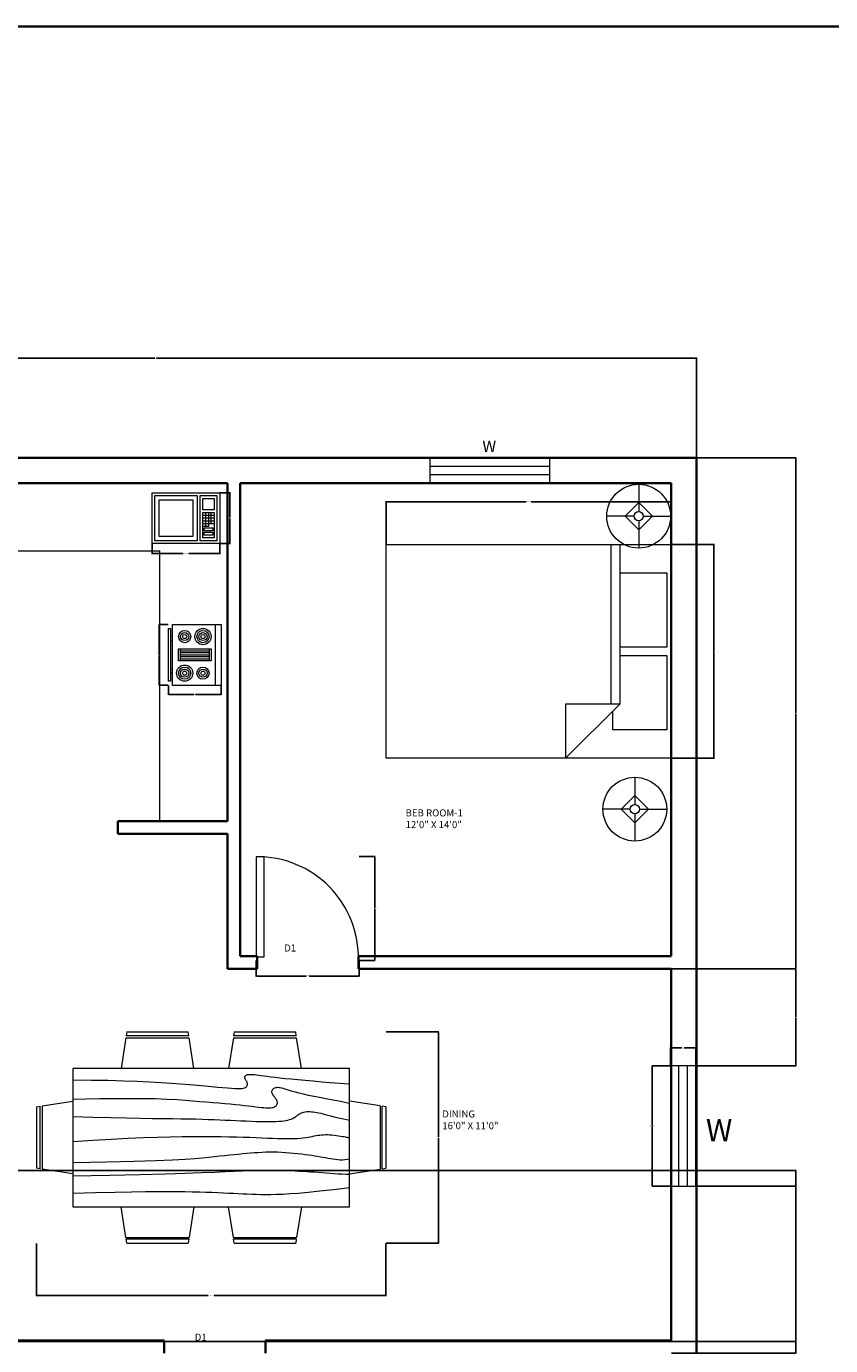
# Model space of a CAD drawing. Units: inches. Extents: x 65 to 1274, y 42 to 1041.
# Tile 3 of 6: x 393 to 678, y 573 to 1041. Entities that reach past the tile are written whole.
import ezdxf

# ---------------------------------------------------------------- set-up
doc = ezdxf.new("R2010")
doc.units = ezdxf.units.IN
for name, color, linetype, lineweight in [('A-ANNO-DIMS', 2, 'Continuous', 18), ('A-AREA-IDEN', 7, 'Continuous', 18), ('A-DOOR', 3, 'Continuous', 18), ('A-EQPM', 9, 'Continuous', 18), ('A-FLOR-CASE', 8, 'Continuous', 18), ('A-FURN', 8, 'Continuous', 18), ('A-GLAZ', 4, 'Continuous', 18), ('A-WALL', 7, 'Continuous', 35), ('Text', 7, 'Continuous', 18), ('Title Block', 7, 'Continuous', 35)]:
    doc.layers.add(name, color=color, linetype=linetype, lineweight=lineweight)
doc.styles.get("Standard").update_dxf_attribs({"font": 'arial.ttf'})
doc.dimstyles.get("Standard").update_dxf_attribs({"dimtxt": 0.18, "dimasz": 0.18, "dimexe": 0.18, "dimexo": 0.0625, "dimgap": 0.09, "dimtad": 0, "dimtih": 1, "dimtoh": 1, "dimdec": 4, "dimzin": 0, "dimdsep": 46, "dimtxsty": 'Standard', "dimcen": 0.09, "dimadec": 0, "dimazin": 0, "dimtfac": 1, "dimtdec": 4, "dimtofl": 0, "dimtmove": 0, "dimatfit": 3, "dimfxl": 1, "dimtolj": 1, "dimtzin": 0, "dimarcsym": 0})

# ---------------------------------------------------------------- blocks, each defined once
blk = doc.blocks.new('Dining Set - 36 x 72 in.')
for p, q in [((-22, 27.5), (-22.1562, 26.50042)), ((-22, 27.5), (-6, 27.5)), ((-5.8437, 26.49966), (-6, 27.5)), ((6, 27.5), (5.8438, 26.50042)), ((6, 27.5), (22, 27.5)), ((22.1563, 26.49966), (22, 27.5)), ((-22.2343, 26.00059), (-23.4847, 17.99762)), ((-22.2304, 26), (-5.7608, 26)), ((-5.8416, 26.5), (-22.1534, 26.5)), ((-4.5152, 17.99762), (-5.7655, 25.99926)), ((5.7657, 26.00059), (4.5153, 17.99762)), ((5.7696, 26), (22.2392, 26)), ((22.1584, 26.5), (5.8466, 26.5)), ((23.4848, 17.99762), (22.2345, 25.99926)), ((36, 18), (-36, 18)), ((-36, 18), (-36, -18)), ((36, -18), (36, 18)), ((-45.5, 8), (-44.5004, 8.15617)), ((-45.5, 8), (-45.5, -8)), ((-44.5, -8.15843), (-44.5, 8.15338)), ((-44.0006, 8.23428), (-35.9976, 9.48474)), ((-44, 8.23041), (-44, -8.23915)), ((44.0006, 8.23428), (35.9976, 9.48474)), ((44, 8.23041), (44, -8.23915)), ((44.5, -8.15843), (44.5, 8.15338)), ((45.5, 8), (44.5005, 8.15617)), ((45.5, 8), (45.5, -8)), ((-44.4997, -8.15631), (-45.5, -8)), ((-35.9976, -9.48476), (-43.9993, -8.2345)), ((35.9976, -9.48476), (43.9993, -8.2345)), ((44.4997, -8.15631), (45.5, -8)), ((-36, -18), (36, -18)), ((-22.2343, -26.0006), (-23.4847, -17.99762)), ((-4.5152, -17.99762), (-5.7655, -25.99928)), ((5.7657, -26.0006), (4.5153, -17.99762)), ((23.4848, -17.99762), (22.2345, -25.99928)), ((-22.2304, -26), (-5.7608, -26)), ((-22, -27.5), (-22.1562, -26.50044)), ((-5.8416, -26.5), (-22.1534, -26.5)), ((-5.8437, -26.49967), (-6, -27.5)), ((5.7696, -26), (22.2392, -26)), ((6, -27.5), (5.8438, -26.50044)), ((22.1584, -26.5), (5.8466, -26.5)), ((22.1563, -26.49967), (22, -27.5)), ((-22, -27.5), (-6, -27.5)), ((6, -27.5), (22, -27.5))]:
    blk.add_line(p, q)
for points in [[(-36, 15), (-31.1772, 14.97754), (-26.8079, 14.91406), (-22.8538, 14.81543), (-19.276, 14.6875), (-16.0362, 14.53613), (-13.0957, 14.36718), (-10.4159, 14.18652), (-7.9583, 14), (-5.6904, 13.81315), (-3.6035, 13.63021), (-1.6954, 13.45508), (0.0365, 13.29166), (1.5945, 13.14388), (2.9811, 13.01562), (4.1988, 12.9108), (5.25, 12.83333), (6.1393, 12.78613), (6.8802, 12.76823), (7.4883, 12.77767), (7.9792, 12.8125), (8.3685, 12.87077), (8.6719, 12.95052), (8.9049, 13.0498), (9.0833, 13.16666), (9.2205, 13.29899), (9.3216, 13.44401), (9.3895, 13.59879), (9.4271, 13.76041), (9.4373, 13.92594), (9.4232, 14.09245), (9.3875, 14.257), (9.3333, 14.41666), (9.2638, 14.56917), (9.1836, 14.71484), (9.0975, 14.85465), (9.0104, 14.98958), (8.9272, 15.1206), (8.8529, 15.2487), (8.7922, 15.37483), (8.75, 15.5), (8.7305, 15.62467), (8.7344, 15.74739), (8.7617, 15.86621), (8.8125, 15.97916), (8.8867, 16.08431), (8.9844, 16.17968), (9.1055, 16.26334), (9.25, 16.33333), (9.4189, 16.38802), (9.6172, 16.42708), (9.8506, 16.45052), (10.125, 16.45833), (10.4463, 16.45052), (10.8203, 16.42708), (11.2529, 16.38802), (11.75, 16.33333), (12.3184, 16.26318), (12.9694, 16.17838), (13.7151, 16.07991), (14.5677, 15.96875), (15.5395, 15.84586), (16.6426, 15.71224), (17.8893, 15.56884), (19.2917, 15.41666), (20.859, 15.25667), (22.5879, 15.08984), (24.4721, 14.91715), (26.5052, 14.73958), (28.6809, 14.5581), (30.9929, 14.3737), (33.4347, 14.18733), (36, 14)], [(-36, 10), (-28.9766, 10.14274), (-23.1725, 10.20442), (-18.4241, 10.19775), (-14.5677, 10.13541), (-11.4399, 10.03011), (-8.877, 9.89453), (-6.7154, 9.74137), (-4.7917, 9.58333), (-2.9698, 9.43082), (-1.2246, 9.28515), (0.4415, 9.14534), (2.026, 9.01041), (3.5266, 8.87939), (4.9408, 8.7513), (6.266, 8.62516), (7.5, 8.5), (8.6411, 8.37549), (9.6914, 8.2539), (10.6538, 8.13818), (11.5312, 8.03125), (12.3267, 7.93603), (13.043, 7.85547), (13.6831, 7.79248), (14.25, 7.75), (14.7471, 7.7303), (15.1797, 7.73307), (15.5537, 7.75732), (15.875, 7.80208), (16.1494, 7.86637), (16.3828, 7.94922), (16.5811, 8.04964), (16.75, 8.16666), (16.8944, 8.29915), (17.0143, 8.44531), (17.1089, 8.60319), (17.1771, 8.77083), (17.218, 8.94629), (17.2305, 9.1276), (17.2137, 9.31282), (17.1667, 9.5), (17.0895, 9.6875), (16.987, 9.875), (16.8649, 10.0625), (16.7292, 10.25), (16.5856, 10.4375), (16.4401, 10.625), (16.2985, 10.8125), (16.1667, 11), (16.05, 11.18733), (15.9518, 11.3737), (15.8752, 11.5581), (15.8229, 11.73958), (15.798, 11.91715), (15.8034, 12.08984), (15.842, 12.25667), (15.9167, 12.41666), (16.0295, 12.56836), (16.1784, 12.70833), (16.3605, 12.83268), (16.5729, 12.9375), (16.8127, 13.01888), (17.0768, 13.07291), (17.3625, 13.0957), (17.6667, 13.08333), (17.9894, 13.03312), (18.3418, 12.94726), (18.7382, 12.82918), (19.1927, 12.68229), (19.7195, 12.51001), (20.3327, 12.31575), (21.0465, 12.10294), (21.875, 11.875), (22.8357, 11.63354), (23.959, 11.37304), (25.2786, 11.08618), (26.8282, 10.76562), (28.6414, 10.40405), (30.752, 9.99414), (33.1936, 9.52856), (36, 9)], [(-36, 5.5), (-30.7157, 5.3348), (-26.069, 5.20963), (-21.9946, 5.11767), (-18.4271, 5.05208), (-15.3009, 5.00602), (-12.5508, 4.97265), (-10.1112, 4.94515), (-7.9167, 4.91666), (-5.909, 4.88167), (-4.0586, 4.83984), (-2.3429, 4.79215), (-0.7396, 4.73958), (0.7739, 4.6831), (2.22, 4.6237), (3.6213, 4.56233), (5, 4.5), (6.373, 4.43782), (7.7344, 4.3776), (9.0723, 4.32129), (10.375, 4.27083), (11.6309, 4.22819), (12.8281, 4.19531), (13.9551, 4.17415), (15, 4.16666), (15.954, 4.17448), (16.819, 4.19791), (17.6001, 4.23698), (18.3021, 4.29166), (18.9299, 4.36198), (19.4883, 4.44791), (19.9823, 4.54948), (20.4167, 4.66666), (20.7969, 4.79899), (21.1302, 4.94401), (21.4245, 5.09879), (21.6875, 5.26041), (21.9271, 5.42594), (22.1511, 5.59245), (22.3672, 5.757), (22.5834, 5.91666), (22.8065, 6.06868), (23.0404, 6.21093), (23.2879, 6.34147), (23.5521, 6.45833), (23.8358, 6.55957), (24.142, 6.64323), (24.4735, 6.70735), (24.8334, 6.75), (25.2235, 6.76969), (25.642, 6.76692), (26.0858, 6.74267), (26.5521, 6.69791), (27.0379, 6.63362), (27.5404, 6.55078), (28.0565, 6.45036), (28.5834, 6.33333), (29.1242, 6.19987), (29.7071, 6.04687), (30.3661, 5.87044), (31.1354, 5.66666), (32.0493, 5.43164), (33.142, 5.16146), (34.4475, 4.85221), (36, 4.5)], [(-36, -1), (-30.7915, -0.6591), (-26.0195, -0.38216), (-21.6519, -0.16284), (-17.6563, 0.00521), (-14.0005, 0.12833), (-10.6523, 0.21289), (-7.5796, 0.26522), (-4.75, 0.29166), (-2.134, 0.29793), (0.2878, 0.28711), (2.5317, 0.26163), (4.6146, 0.22396), (6.5529, 0.17651), (8.3633, 0.12174), (10.0623, 0.06209), (11.6667, 0), (13.1899, -0.06201), (14.6341, -0.1211), (15.9982, -0.17432), (17.2813, -0.21875), (18.4823, -0.25147), (19.6003, -0.26953), (20.6343, -0.27002), (21.5834, -0.25), (22.4481, -0.20768), (23.2357, -0.14584), (23.9549, -0.06836), (24.6146, 0.02083), (25.2235, 0.11784), (25.7904, 0.21875), (26.3241, 0.31966), (26.8334, 0.41666), (27.3265, 0.50618), (27.8099, 0.58593), (28.2894, 0.65397), (28.7709, 0.70833), (29.2601, 0.74707), (29.763, 0.76823), (30.2855, 0.76985), (30.8334, 0.75), (31.4088, 0.70784), (31.9994, 0.64713), (32.589, 0.57275), (33.1615, 0.48958), (33.7008, 0.4025), (34.1908, 0.3164), (34.6153, 0.23616), (34.9584, 0.16666), (35.2099, 0.11165), (35.3848, 0.07031), (35.504, 0.04069), (35.5886, 0.02083), (35.6594, 0.00879), (35.7377, 0.0026), (35.8442, 0.00032), (36, 0)], [(-36, -6.5), (-27.1843, -6.31267), (-20.084, -6.1263), (-14.469, -5.9419), (-10.1094, -5.76042), (-6.7752, -5.58285), (-4.2363, -5.41016), (-2.2629, -5.24333), (-0.625, -5.08334), (0.8708, -4.93099), (2.2715, -4.78646), (3.5872, -4.64974), (4.8281, -4.52084), (6.0046, -4.39974), (7.127, -4.28646), (8.2053, -4.18099), (9.25, -4.08334), (10.2705, -3.99382), (11.2734, -3.91407), (12.2647, -3.84603), (13.25, -3.79167), (14.2354, -3.75293), (15.2266, -3.73177), (16.2295, -3.73015), (17.25, -3.75), (18.2912, -3.79248), (19.3451, -3.85547), (20.4009, -3.93604), (21.4479, -4.03125), (22.4754, -4.13819), (23.4727, -4.25391), (24.4289, -4.37549), (25.3334, -4.5), (26.1785, -4.62492), (26.9694, -4.74935), (27.7145, -4.87281), (28.4219, -4.99479), (29.1, -5.11483), (29.7572, -5.23242), (30.4016, -5.34709), (31.0417, -5.45834), (31.6837, -5.56437), (32.3262, -5.65821), (32.9658, -5.73153), (33.599, -5.77604), (34.2224, -5.78345), (34.8327, -5.74545), (35.4264, -5.65373), (36, -5.5)], [(-36, -10), (-26.4022, -9.81299), (-18.4675, -9.62891), (-11.9839, -9.45069), (-6.7396, -9.28125), (-2.5226, -9.12354), (0.8789, -8.98047), (3.6769, -8.85498), (6.0833, -8.75), (8.2767, -8.66765), (10.3021, -8.60677), (12.1712, -8.56543), (13.8958, -8.54167), (15.4876, -8.53353), (16.9583, -8.53907), (18.3197, -8.55632), (19.5834, -8.58334), (20.7616, -8.61841), (21.8685, -8.66081), (22.9188, -8.71004), (23.9271, -8.76563), (24.9081, -8.82707), (25.8763, -8.89388), (26.8465, -8.96558), (27.8334, -9.04167), (28.8474, -9.12118), (29.8828, -9.20117), (30.93, -9.27824), (31.9792, -9.34896), (33.0205, -9.40991), (34.0443, -9.45768), (35.0407, -9.48885), (36, -9.5)], [(-36, -14.5), (-30.0881, -14.33513), (-25.0332, -14.21224), (-20.7312, -14.12647), (-17.0781, -14.07292), (-13.97, -14.04671), (-11.3027, -14.04297), (-8.9724, -14.05681), (-6.875, -14.08334), (-4.9224, -14.11833), (-3.0905, -14.16016), (-1.3709, -14.20785), (0.2448, -14.26042), (1.7647, -14.3169), (3.1973, -14.3763), (4.5507, -14.43767), (5.8333, -14.5), (7.0554, -14.5621), (8.235, -14.62175), (9.3922, -14.67652), (10.5469, -14.72396), (11.7192, -14.76164), (12.929, -14.78711), (14.1965, -14.79794), (15.5417, -14.79167), (16.9933, -14.76424), (18.6152, -14.70508), (20.4804, -14.60197), (22.6615, -14.44271), (25.2312, -14.21509), (28.2624, -13.9069), (31.8277, -13.50594), (36, -13)]]:
    blk.add_lwpolyline(points)
blk = doc.blocks.new('Range-Oven - 30 in top')
for p, q in [((0, -3), (30, -3)), ((12, -6), (18, -6)), ((13, -20), (13, -6)), ((14, -6), (14, -20)), ((15, -20), (15, -6)), ((16, -6), (16, -20)), ((17, -20), (17, -6)), ((6, -24), (6, -25)), ((8, -25), (8, -24)), ((18, -20), (12, -20)), ((22, -25), (22, -24)), ((24, -24), (24, -25))]:
    blk.add_line(p, q)
for points in [[(0, -24), (0, 0), (30, 0), (30, -24)], [(12, -21), (12, -5), (18, -5), (18, -21)], [(2, -26), (2, -25), (28, -25), (28, -26)]]:
    blk.add_lwpolyline(points, close=True)
for centre, radius in [((6, -9), 4), ((6, -9), 3), ((24, -9), 3), ((6, -9), 2), ((6, -9), 1), ((24, -9), 2), ((24, -9), 1), ((6, -18), 3), ((6, -18), 2), ((6, -18), 1), ((24, -18), 4), ((24, -18), 3), ((24, -18), 2), ((24, -18), 1)]:
    blk.add_circle(centre, radius)
blk = doc.blocks.new('Bed - Queen')
for p, q in [((0, -80.00003), (0, 0)), ((0, 0), (59.99999, 0)), ((59.99999, 0), (59.99999, -80.00003)), ((7.99999, -1.2), (28.79998, -1.2)), ((7.99999, -14.4), (7.99999, -1.2)), ((28.79998, -1.2), (28.79998, -14.4)), ((31.19999, -1.2), (51.99999, -1.2)), ((31.19999, -14.4), (31.19999, -1.2)), ((51.99999, -1.2), (51.99999, -16.4)), ((0, -14.4), (44.8, -14.4)), ((59.99999, -29.6), (44.8, -14.4)), ((44.8, -14.4), (44.8, -29.6)), ((44.8, -16.8), (0, -16.8)), ((51.99999, -16.4), (46.79936, -16.4)), ((44.8, -29.6), (59.99999, -29.6)), ((59.99999, -80.00003), (0, -80.00003))]:
    blk.add_line(p, q)
blk = doc.blocks.new('Microwave')
for p, q in [((18, 10), (22, 10)), ((19, 7), (19, 11)), ((20, 11), (20, 7)), ((21, 7), (21, 11)), ((22, 9), (18, 9)), ((18, 8), (22, 8)), ((22, 7), (18, 7)), ((20, 6), (18, 6)), ((19, 6), (19, 7)), ((20, 7), (20, 6))]:
    blk.add_line(p, q)
for points in [[(0, 0), (0, 18), (24, 18), (24, 0)], [(1, 1), (1, 17), (16, 17), (16, 1)], [(2.5, 2.5), (2.5, 15.5), (14.5, 15.5), (14.5, 2.5)], [(17, 1), (17, 17), (23, 17), (23, 1)], [(18, 12), (18, 16), (22, 16), (22, 12)], [(18, 2), (18, 11), (22, 11), (22, 2)], [(18.5, 4.5), (18.5, 5.5), (21.5, 5.5), (21.5, 4.5)], [(18.5, 3), (18.5, 4), (21.5, 4), (21.5, 3)]]:
    blk.add_lwpolyline(points, close=True)
blk = doc.blocks.new('Lamp - Table')
for p, q in [((0, 7), (0, 1)), ((0, 3), (-3, 0)), ((3, 0), (0, 3)), ((-1, 0), (-7, 0)), ((-3, 0), (0, -3)), ((0, -3), (3, 0)), ((1, 0), (7, 0)), ((0, -1), (0, -7))]:
    blk.add_line(p, q)
for radius in [7, 1]:
    blk.add_circle((0, 0), radius)
blk = doc.blocks.new('WIN-43-DEEP-FRAME')
for p, q in [((9, 42.65), (0, 42.65)), ((0, 42.65), (0, 0)), ((3, 0), (3, 42.65)), ((6, 42.65), (6, 0)), ((9, 0), (9, 42.65)), ((0, 0), (9, 0))]:
    blk.add_line(p, q)
blk = doc.blocks.new('DOOR-SINGLE-36')
blk.add_lwpolyline([(0.01, 1.25), (2.82, 1.25), (2.82, 36.75), (0.01, 36.75)], close=True)
blk.add_arc((0.35, 0.95), 35.9, 358.4887, 90.5615)
blk = doc.blocks.new('*D20')
at = {"layer": 'A-ANNO-DIMS', "color": 0, "lineweight": -2, "transparency": 16777216}
for p, q in [((621.33, 672.11), (614.81, 672.11)), ((614.99, 671.93), (614.99, 650.97)), ((614.99, 629.64), (614.99, 650.6)), ((621.33, 629.46), (614.81, 629.46))]:
    blk.add_line(p, q, dxfattribs=at)
at = {"layer": 'A-ANNO-DIMS', "color": 0, "transparency": 16777216}
for points in [[(614.96, 671.93), (615.02, 671.93), (614.99, 672.11)], [(614.96, 629.64), (615.02, 629.64), (614.99, 629.46)]]:
    blk.add_solid(points, dxfattribs=at)
at = {"layer": 'Defpoints', "color": 0, "transparency": 16777216}
for p in [(621.39, 672.11), (614.99, 629.46), (621.39, 629.46)]:
    blk.add_point(p, dxfattribs=at)
at = {"layer": 'A-ANNO-DIMS', "color": 0, "transparency": 16777216, "insert": (614.99, 650.78), "char_height": 0.18, "attachment_point": 5}
blk.add_mtext('\\A1;WINDOW 43 TYP.', dxfattribs=at)
blk = doc.blocks.new('*D21')
at = {"layer": 'A-ANNO-DIMS', "color": 0, "lineweight": -2, "transparency": 16777216}
for p, q in [((621.39, 672.17), (621.39, 678.69)), ((621.57, 678.51), (625.43, 678.51)), ((630.21, 678.51), (626.35, 678.51)), ((630.39, 672.17), (630.39, 678.69))]:
    blk.add_line(p, q, dxfattribs=at)
at = {"layer": 'A-ANNO-DIMS', "color": 0, "transparency": 16777216}
for points in [[(621.57, 678.54), (621.57, 678.48), (621.39, 678.51)], [(630.21, 678.54), (630.21, 678.48), (630.39, 678.51)]]:
    blk.add_solid(points, dxfattribs=at)
at = {"layer": 'Defpoints', "color": 0, "transparency": 16777216}
for p in [(621.39, 678.51), (621.39, 672.11), (630.39, 672.11)]:
    blk.add_point(p, dxfattribs=at)
at = {"layer": 'A-ANNO-DIMS', "color": 0, "transparency": 16777216, "insert": (625.89, 678.51), "char_height": 0.18, "attachment_point": 5}
blk.add_mtext('\\A1;9 TYP.', dxfattribs=at)
blk = doc.blocks.new('*D24')
at = {"layer": 'A-ANNO-DIMS', "color": 0, "lineweight": -2, "transparency": 16777216}
for p, q in [((510.95, 746.54), (516.61, 746.54)), ((516.43, 746.36), (516.43, 728.25)), ((516.43, 709.77), (516.43, 727.88)), ((510.95, 709.59), (516.61, 709.59))]:
    blk.add_line(p, q, dxfattribs=at)
at = {"layer": 'A-ANNO-DIMS', "color": 0, "transparency": 16777216}
for points in [[(516.4, 746.36), (516.46, 746.36), (516.43, 746.54)], [(516.4, 709.77), (516.46, 709.77), (516.43, 709.59)]]:
    blk.add_solid(points, dxfattribs=at)
at = {"layer": 'Defpoints', "color": 0, "transparency": 16777216}
for p in [(510.89, 746.54), (516.43, 746.54), (510.89, 709.59)]:
    blk.add_point(p, dxfattribs=at)
at = {"layer": 'A-ANNO-DIMS', "color": 0, "transparency": 16777216, "insert": (516.43, 728.06), "char_height": 0.18, "attachment_point": 5}
blk.add_mtext('\\A1;ROOM DOOR 37 TYP.', dxfattribs=at)
blk = doc.blocks.new('*D25')
at = {"layer": 'A-ANNO-DIMS', "color": 0, "lineweight": -2, "transparency": 16777216}
for p, q in [((474.39, 709.53), (474.39, 703.87)), ((510.89, 709.53), (510.89, 703.87)), ((474.57, 704.05), (492.11, 704.05)), ((510.71, 704.05), (493.17, 704.05))]:
    blk.add_line(p, q, dxfattribs=at)
at = {"layer": 'A-ANNO-DIMS', "color": 0, "transparency": 16777216}
for points in [[(474.57, 704.08), (474.57, 704.02), (474.39, 704.05)], [(510.71, 704.08), (510.71, 704.02), (510.89, 704.05)]]:
    blk.add_solid(points, dxfattribs=at)
at = {"layer": 'Defpoints', "color": 0, "transparency": 16777216}
for p in [(474.39, 709.59), (510.89, 709.59), (510.89, 704.05)]:
    blk.add_point(p, dxfattribs=at)
at = {"layer": 'A-ANNO-DIMS', "color": 0, "transparency": 16777216, "insert": (492.64, 704.05), "char_height": 0.18, "attachment_point": 5}
blk.add_mtext('\\A1;36 TYP.', dxfattribs=at)
blk = doc.blocks.new('*D28')
at = {"layer": 'A-ANNO-DIMS', "color": 0, "lineweight": -2, "transparency": 16777216}
for p, q in [((520.48, 857.36), (520.48, 872.66)), ((520.66, 872.48), (570.18, 872.48)), ((621.48, 872.48), (571.96, 872.48)), ((621.66, 857.36), (621.66, 872.66))]:
    blk.add_line(p, q, dxfattribs=at)
at = {"layer": 'A-ANNO-DIMS', "color": 0, "transparency": 16777216}
for points in [[(520.66, 872.51), (520.66, 872.45), (520.48, 872.48)], [(621.48, 872.51), (621.48, 872.45), (621.66, 872.48)]]:
    blk.add_solid(points, dxfattribs=at)
at = {"layer": 'Defpoints', "color": 0, "transparency": 16777216}
for p in [(621.66, 872.48), (520.48, 857.3), (621.66, 857.3)]:
    blk.add_point(p, dxfattribs=at)
at = {"layer": 'A-ANNO-DIMS', "color": 0, "transparency": 16777216, "insert": (571.07, 872.48), "char_height": 0.18, "attachment_point": 5}
blk.add_mtext('\\A1;BED 101 TYP.', dxfattribs=at)
blk = doc.blocks.new('*D29')
at = {"layer": 'A-ANNO-DIMS', "color": 0, "lineweight": -2, "transparency": 16777216}
for p, q in [((621.72, 857.3), (637.01, 857.3)), ((636.83, 857.12), (636.83, 819.54)), ((636.83, 781.6), (636.83, 819.18)), ((621.72, 781.42), (637.01, 781.42))]:
    blk.add_line(p, q, dxfattribs=at)
at = {"layer": 'A-ANNO-DIMS', "color": 0, "transparency": 16777216}
for points in [[(636.8, 857.12), (636.86, 857.12), (636.83, 857.3)], [(636.8, 781.6), (636.86, 781.6), (636.83, 781.42)]]:
    blk.add_solid(points, dxfattribs=at)
at = {"layer": 'Defpoints', "color": 0, "transparency": 16777216}
for p in [(621.66, 857.3), (621.66, 781.42), (636.83, 781.42)]:
    blk.add_point(p, dxfattribs=at)
at = {"layer": 'A-ANNO-DIMS', "color": 0, "transparency": 16777216, "insert": (636.83, 819.36), "char_height": 0.18, "attachment_point": 5}
blk.add_mtext('\\A1;76 TYP.', dxfattribs=at)
blk = doc.blocks.new('*D44')
at = {"layer": 'A-ANNO-DIMS', "color": 0, "lineweight": -2, "transparency": 16777216}
for p, q in [((396.34, 609.13), (396.34, 590.4)), ((520.42, 609.13), (520.42, 590.4)), ((396.52, 590.58), (457.34, 590.58)), ((520.24, 590.58), (459.42, 590.58))]:
    blk.add_line(p, q, dxfattribs=at)
at = {"layer": 'A-ANNO-DIMS', "color": 0, "transparency": 16777216}
for points in [[(396.52, 590.61), (396.52, 590.55), (396.34, 590.58)], [(520.24, 590.61), (520.24, 590.55), (520.42, 590.58)]]:
    blk.add_solid(points, dxfattribs=at)
at = {"layer": 'Defpoints', "color": 0, "transparency": 16777216}
for p in [(396.34, 609.19), (520.42, 609.19), (520.42, 590.58)]:
    blk.add_point(p, dxfattribs=at)
at = {"layer": 'A-ANNO-DIMS', "color": 0, "transparency": 16777216, "insert": (458.38, 590.58), "char_height": 0.18, "attachment_point": 5}
blk.add_mtext('\\A1;DINING SET 124', dxfattribs=at)
blk = doc.blocks.new('*D45')
at = {"layer": 'A-ANNO-DIMS', "color": 0, "lineweight": -2, "transparency": 16777216}
for p, q in [((520.48, 684.19), (539.21, 684.19)), ((539.03, 684.01), (539.03, 646.87)), ((539.03, 609.37), (539.03, 646.51)), ((520.48, 609.19), (539.21, 609.19))]:
    blk.add_line(p, q, dxfattribs=at)
at = {"layer": 'A-ANNO-DIMS', "color": 0, "transparency": 16777216}
for points in [[(539, 684.01), (539.06, 684.01), (539.03, 684.19)], [(539, 609.37), (539.06, 609.37), (539.03, 609.19)]]:
    blk.add_solid(points, dxfattribs=at)
at = {"layer": 'Defpoints', "color": 0, "transparency": 16777216}
for p in [(520.42, 684.19), (539.03, 684.19), (520.42, 609.19)]:
    blk.add_point(p, dxfattribs=at)
at = {"layer": 'A-ANNO-DIMS', "color": 0, "transparency": 16777216, "insert": (539.03, 646.69), "char_height": 0.18, "attachment_point": 5}
blk.add_mtext('\\A1;75', dxfattribs=at)
blk = doc.blocks.new('*D46')
at = {"layer": 'A-ANNO-DIMS', "color": 0, "lineweight": -2, "transparency": 16777216}
for p, q in [((443.13, 828.92), (439.77, 828.92)), ((439.95, 828.74), (439.95, 818.29)), ((439.95, 807.47), (439.95, 817.92)), ((443.13, 807.29), (439.77, 807.29))]:
    blk.add_line(p, q, dxfattribs=at)
at = {"layer": 'A-ANNO-DIMS', "color": 0, "transparency": 16777216}
for points in [[(439.92, 828.74), (439.98, 828.74), (439.95, 828.92)], [(439.92, 807.47), (439.98, 807.47), (439.95, 807.29)]]:
    blk.add_solid(points, dxfattribs=at)
at = {"layer": 'Defpoints', "color": 0, "transparency": 16777216}
for p in [(443.19, 828.92), (439.95, 807.29), (443.19, 807.29)]:
    blk.add_point(p, dxfattribs=at)
at = {"layer": 'A-ANNO-DIMS', "color": 0, "transparency": 16777216, "insert": (439.95, 818.11), "char_height": 0.18, "attachment_point": 5}
blk.add_mtext('\\A1;RANGE 22', dxfattribs=at)
blk = doc.blocks.new('*D47')
at = {"layer": 'A-ANNO-DIMS', "color": 0, "lineweight": -2, "transparency": 16777216}
for p, q in [((443.19, 807.22), (443.19, 803.86)), ((461.95, 807.22), (461.95, 803.86)), ((443.37, 804.04), (452.36, 804.04)), ((461.77, 804.04), (452.78, 804.04))]:
    blk.add_line(p, q, dxfattribs=at)
at = {"layer": 'A-ANNO-DIMS', "color": 0, "transparency": 16777216}
for points in [[(443.37, 804.07), (443.37, 804.01), (443.19, 804.04)], [(461.77, 804.07), (461.77, 804.01), (461.95, 804.04)]]:
    blk.add_solid(points, dxfattribs=at)
at = {"layer": 'Defpoints', "color": 0, "transparency": 16777216}
for p in [(443.19, 807.29), (461.95, 807.29), (461.95, 804.04)]:
    blk.add_point(p, dxfattribs=at)
at = {"layer": 'A-ANNO-DIMS', "color": 0, "transparency": 16777216, "insert": (452.57, 804.04), "char_height": 0.18, "attachment_point": 5}
blk.add_mtext('\\A1;19', dxfattribs=at)
blk = doc.blocks.new('*D48')
at = {"layer": 'A-ANNO-DIMS', "color": 0, "lineweight": -2, "transparency": 16777216}
for p, q in [((437.41, 857.6), (437.41, 853.88)), ((461.41, 857.6), (461.41, 853.88)), ((437.59, 854.06), (448.37, 854.06)), ((461.23, 854.06), (450.45, 854.06))]:
    blk.add_line(p, q, dxfattribs=at)
at = {"layer": 'A-ANNO-DIMS', "color": 0, "transparency": 16777216}
for points in [[(437.59, 854.09), (437.59, 854.03), (437.41, 854.06)], [(461.23, 854.09), (461.23, 854.03), (461.41, 854.06)]]:
    blk.add_solid(points, dxfattribs=at)
at = {"layer": 'Defpoints', "color": 0, "transparency": 16777216}
for p in [(437.41, 857.66), (461.41, 857.66), (461.41, 854.06)]:
    blk.add_point(p, dxfattribs=at)
at = {"layer": 'A-ANNO-DIMS', "color": 0, "transparency": 16777216, "insert": (449.41, 854.06), "char_height": 0.18, "attachment_point": 5}
blk.add_mtext('\\A1;MICROWAVE 24', dxfattribs=at)
blk = doc.blocks.new('*D49')
at = {"layer": 'A-ANNO-DIMS', "color": 0, "lineweight": -2, "transparency": 16777216}
for p, q in [((461.48, 875.66), (465.19, 875.66)), ((465.01, 875.48), (465.01, 866.84)), ((465.01, 857.84), (465.01, 866.48)), ((461.48, 857.66), (465.19, 857.66))]:
    blk.add_line(p, q, dxfattribs=at)
at = {"layer": 'A-ANNO-DIMS', "color": 0, "transparency": 16777216}
for points in [[(464.98, 875.48), (465.04, 875.48), (465.01, 875.66)], [(464.98, 857.84), (465.04, 857.84), (465.01, 857.66)]]:
    blk.add_solid(points, dxfattribs=at)
at = {"layer": 'Defpoints', "color": 0, "transparency": 16777216}
for p in [(461.41, 875.66), (465.01, 875.66), (461.41, 857.66)]:
    blk.add_point(p, dxfattribs=at)
at = {"layer": 'A-ANNO-DIMS', "color": 0, "transparency": 16777216, "insert": (465.01, 866.66), "char_height": 0.18, "attachment_point": 5}
blk.add_mtext('\\A1;18', dxfattribs=at)
blk = doc.blocks.new('*D52')
at = {"layer": 'A-ANNO-DIMS', "color": 0, "lineweight": -2, "transparency": 16777216}
for p, q in [((246.69, 888.16), (246.69, 923.68)), ((246.87, 923.5), (438.4, 923.5)), ((630.51, 923.5), (438.98, 923.5)), ((630.69, 888.16), (630.69, 923.68))]:
    blk.add_line(p, q, dxfattribs=at)
at = {"layer": 'A-ANNO-DIMS', "color": 0, "transparency": 16777216}
for points in [[(246.87, 923.53), (246.87, 923.47), (246.69, 923.5)], [(630.51, 923.53), (630.51, 923.47), (630.69, 923.5)]]:
    blk.add_solid(points, dxfattribs=at)
at = {"layer": 'Defpoints', "color": 0, "transparency": 16777216}
for p in [(630.69, 923.5), (246.69, 888.1), (630.69, 888.1)]:
    blk.add_point(p, dxfattribs=at)
at = {"layer": 'A-ANNO-DIMS', "color": 0, "transparency": 16777216, "insert": (438.69, 923.5), "char_height": 0.18, "attachment_point": 5}
blk.add_mtext('\\A1;384', dxfattribs=at)
blk = doc.blocks.new('*D59')
at = {"layer": 'A-ANNO-DIMS', "color": 0, "lineweight": -2, "transparency": 16777216}
for p, q in [((630.45, 629.46), (666.07, 629.46)), ((665.89, 629.28), (665.89, 599.96)), ((665.89, 570.28), (665.89, 599.6)), ((621.75, 570.1), (666.07, 570.1))]:
    blk.add_line(p, q, dxfattribs=at)
at = {"layer": 'A-ANNO-DIMS', "color": 0, "transparency": 16777216}
for points in [[(665.86, 629.28), (665.92, 629.28), (665.89, 629.46)], [(665.86, 570.28), (665.92, 570.28), (665.89, 570.1)]]:
    blk.add_solid(points, dxfattribs=at)
at = {"layer": 'Defpoints', "color": 0, "transparency": 16777216}
for p in [(630.39, 629.46), (665.89, 629.46), (621.69, 570.1)]:
    blk.add_point(p, dxfattribs=at)
at = {"layer": 'A-ANNO-DIMS', "color": 0, "transparency": 16777216, "insert": (665.89, 599.78), "char_height": 0.18, "attachment_point": 5}
blk.add_mtext('\\A1;59.36', dxfattribs=at)
blk = doc.blocks.new('*D60')
at = {"layer": 'A-ANNO-DIMS', "color": 0, "lineweight": -2, "transparency": 16777216}
for p, q in [((621.75, 706.6), (666.07, 706.6)), ((665.89, 706.42), (665.89, 689.54)), ((665.89, 672.29), (665.89, 689.17)), ((630.45, 672.11), (666.07, 672.11))]:
    blk.add_line(p, q, dxfattribs=at)
at = {"layer": 'A-ANNO-DIMS', "color": 0, "transparency": 16777216}
for points in [[(665.86, 706.42), (665.92, 706.42), (665.89, 706.6)], [(665.86, 672.29), (665.92, 672.29), (665.89, 672.11)]]:
    blk.add_solid(points, dxfattribs=at)
at = {"layer": 'Defpoints', "color": 0, "transparency": 16777216}
for p in [(621.69, 706.6), (665.89, 706.6), (630.39, 672.11)]:
    blk.add_point(p, dxfattribs=at)
at = {"layer": 'A-ANNO-DIMS', "color": 0, "transparency": 16777216, "insert": (665.89, 689.35), "char_height": 0.18, "attachment_point": 5}
blk.add_mtext('\\A1;34.49', dxfattribs=at)
blk = doc.blocks.new('*D61')
at = {"layer": 'A-ANNO-DIMS', "color": 0, "lineweight": -2, "transparency": 16777216}
for p, q in [((630.75, 888.1), (666.07, 888.1)), ((665.89, 887.92), (665.89, 797.53)), ((665.89, 706.78), (665.89, 797.17)), ((621.75, 706.6), (666.07, 706.6))]:
    blk.add_line(p, q, dxfattribs=at)
at = {"layer": 'A-ANNO-DIMS', "color": 0, "transparency": 16777216}
for points in [[(665.86, 887.92), (665.92, 887.92), (665.89, 888.1)], [(665.86, 706.78), (665.92, 706.78), (665.89, 706.6)]]:
    blk.add_solid(points, dxfattribs=at)
at = {"layer": 'Defpoints', "color": 0, "transparency": 16777216}
for p in [(630.69, 888.1), (665.89, 888.1), (621.69, 706.6)]:
    blk.add_point(p, dxfattribs=at)
at = {"layer": 'A-ANNO-DIMS', "color": 0, "transparency": 16777216, "insert": (665.89, 797.35), "char_height": 0.18, "attachment_point": 5}
blk.add_mtext('\\A1;181.5', dxfattribs=at)
blk = doc.blocks.new('*D62')
at = {"layer": 'A-ANNO-DIMS', "color": 0, "lineweight": -2, "transparency": 16777216}
for p, q in [((347.47, 635.01), (666.07, 635.01)), ((665.89, 634.83), (665.89, 604.83)), ((665.89, 574.45), (665.89, 604.46)), ((347.47, 574.27), (666.07, 574.27))]:
    blk.add_line(p, q, dxfattribs=at)
at = {"layer": 'A-ANNO-DIMS', "color": 0, "transparency": 16777216}
for points in [[(665.86, 634.83), (665.92, 634.83), (665.89, 635.01)], [(665.86, 574.45), (665.92, 574.45), (665.89, 574.27)]]:
    blk.add_solid(points, dxfattribs=at)
at = {"layer": 'Defpoints', "color": 0, "transparency": 16777216}
for p in [(347.41, 635.01), (665.89, 635.01), (347.41, 574.27)]:
    blk.add_point(p, dxfattribs=at)
at = {"layer": 'A-ANNO-DIMS', "color": 0, "transparency": 16777216, "insert": (665.89, 604.64), "char_height": 0.18, "attachment_point": 5}
blk.add_mtext('\\A1;60.74', dxfattribs=at)

msp = doc.modelspace()

# ---------------------------------------------------------------- linework, layer by layer
at = {"layer": 'A-FLOR-CASE'}
for p in [(320.1872, 855.1013), (440.1872, 759.1013)]:
    msp.add_line(p, (440.1872, 855.1013), dxfattribs=at)
at = {"layer": 'A-WALL'}
for p, q in [((246.6872, 888.1013), (630.6872, 888.1013)), ((630.6872, 888.1013), (630.6872, 231.1013)), ((320.1872, 879.1013), (464.1872, 879.1013)), ((464.1872, 759.1013), (464.1872, 879.1013)), ((468.6872, 711.1013), (468.6872, 879.1013)), ((468.6872, 879.1013), (621.6872, 879.1013)), ((621.6872, 879.1013), (621.6872, 711.1013)), ((425.1872, 759.1013), (425.1872, 754.6013)), ((425.1872, 759.1013), (464.1872, 759.1013)), ((425.1872, 754.6013), (464.1872, 754.6013)), ((464.1872, 706.6013), (464.1872, 754.6013)), ((468.6872, 711.1013), (474.6872, 711.1013)), ((474.6872, 706.6013), (474.6872, 711.1013)), ((510.6872, 706.6013), (510.6872, 711.1013)), ((510.6872, 711.1013), (621.6872, 711.1013)), ((464.1872, 706.6013), (474.6872, 706.6013)), ((510.6872, 706.6013), (621.6872, 706.6013)), ((621.6872, 706.6013), (621.6872, 574.6013)), ((255.6872, 574.6013), (441.6872, 574.6013)), ((441.6872, 574.6013), (441.6872, 570.1013)), ((477.6872, 574.6013), (477.6872, 570.1013)), ((477.6872, 574.6013), (621.6872, 574.6013))]:
    msp.add_line(p, q, dxfattribs=at)
at = {"layer": 'Title Block'}
msp.add_lwpolyline([(64.7421, 1041.286), (1273.976, 1041.286), (1273.976, 41.6396), (64.7421, 41.6396)], close=True, dxfattribs=at)

# ---------------------------------------------------------------- block references
at = {"layer": 'A-DOOR'}
msp.add_blockref('DOOR-SINGLE-36', (474.389, 709.593), dxfattribs=at)
at = {"layer": 'A-EQPM'}
msp.add_blockref('Microwave', (437.4131, 857.6577), dxfattribs=at)
at = {"layer": 'A-EQPM', "xscale": 0.7212589014959784, "yscale": 0.7212589014959784, "zscale": 0.7212589014959784, "rotation": 270}
msp.add_blockref('Range-Oven - 30 in top', (461.9471, 828.9245), dxfattribs=at)
at = {"layer": 'A-FURN'}
for name, p, xscale, yscale, zscale in [('Lamp - Table', (610.149, 867.3532), 1.619462315136964, 1.619462315136964, 1.619462315136964), ('Lamp - Table', (608.7792, 763.31), 1.619462315136964, 1.619462315136964, 1.619462315136964), ('Dining Set - 36 x 72 in.', (458.3791, 646.6925), 1.363558762198461, 1.363558762198461, 1.363558762198461)]:
    msp.add_blockref(name, p, dxfattribs=dict(at, xscale=xscale, yscale=yscale, zscale=zscale))
at = {"layer": 'A-FURN', "xscale": 1.264723082454659, "yscale": 1.264723082454659, "zscale": 1.264723082454659, "rotation": 270}
msp.add_blockref('Bed - Queen', (621.6576, 857.3021), dxfattribs=at)
at = {"layer": 'A-GLAZ'}
for p, rotation in [((535.9909, 888.075), 270.0000000000003), ((630.3914, 672.1091), 180)]:
    msp.add_blockref('WIN-43-DEEP-FRAME', p, dxfattribs=dict(at, rotation=rotation))

# ---------------------------------------------------------------- texts
at = {"layer": 'A-AREA-IDEN', "char_height": 2.5, "attachment_point": 1}
for s, width, insert in [('BEB ROOM-1\\P12\'0" X 14\'0"', 29.773229, (527.4013, 763.2427)), ('DINING\\P16\'0" X 11\'0"', 42.551509, (540.4119, 656.3207))]:
    msp.add_mtext_dynamic_manual_height_columns(s, width=width, gutter_width=12.5, heights=[0], dxfattribs=dict(at, insert=insert))
at = {"layer": 'Text', "attachment_point": 1}
for s, width, gutter_width, insert, char_height in [('W', 21.242927, 20.3032, (554.6623, 894.1596), 4.0606), ('D1', 11.157779, 12.5, (484.2975, 715.2666), 2.5), ('W', 96.254197, 39.1027, (634.0213, 653.2323), 7.8205), ('D1', 13.983315, 12.5, (452.5325, 577.0506), 2.5)]:
    msp.add_mtext_dynamic_manual_height_columns(s, width=width, gutter_width=gutter_width, heights=[0], dxfattribs=dict(at, insert=insert, char_height=char_height))

# ---------------------------------------------------------------- dimensions: what is measured, and where the dimension line sits
at = {"layer": 'A-ANNO-DIMS'}
for base, p1, p2, picture, middle in [((630.6872, 923.4993), (246.6872, 888.1013), (630.6872, 888.1013), '*D52', (438.6872, 923.4993)), ((461.9471, 804.0411), (443.1943, 807.2868), (461.9471, 807.2868), '*D47', (452.5707, 804.0411))]:
    dim = msp.add_linear_dim(base=base, p1=p1, p2=p2, dimstyle='Standard', override={"dimdec": 0, "dimlfac": 1, "dimrnd": 0, "dimzin": 0, "dimdsep": 46, "dimlunit": 2}, dxfattribs=at)
    dim.commit()
    dim.dimension.update_dxf_attribs({"geometry": picture, "text_midpoint": middle})
for base, p1, p2, override, picture, middle in [((665.8872, 888.1013), (621.6872, 706.6013), (630.6872, 888.1013), {"dimdec": 1, "dimlfac": 1, "dimrnd": 0, "dimzin": 0, "dimdsep": 46, "dimlunit": 2}, '*D61', (665.8872, 797.3513)), ((465.0131, 875.6577), (461.4131, 857.6577), (461.4131, 875.6577), {"dimdec": 0, "dimlfac": 1, "dimrnd": 0, "dimzin": 0, "dimdsep": 46, "dimlunit": 2}, '*D49', (465.0131, 866.6577)), ((665.8872, 706.6013), (630.3914, 672.1086), (621.6872, 706.6013), {"dimdec": 2, "dimlfac": 1, "dimrnd": 0, "dimzin": 0, "dimdsep": 46, "dimlunit": 2}, '*D60', (665.8872, 689.355)), ((539.0336, 684.1904), (520.4211, 609.1946), (520.4211, 684.1904), {"dimdec": 0, "dimlfac": 1, "dimrnd": 0, "dimzin": 0, "dimdsep": 46, "dimlunit": 2}, '*D45', (539.0336, 646.6925)), ((665.8872, 635.0131), (347.4055, 574.2747), (347.4055, 635.0131), {"dimdec": 2, "dimlfac": 1, "dimrnd": 0, "dimzin": 0, "dimdsep": 46, "dimlunit": 2}, '*D62', (665.8872, 604.6439)), ((665.8872, 629.4605), (621.6872, 570.1013), (630.3914, 629.4605), {"dimdec": 2, "dimlfac": 1, "dimrnd": 0, "dimzin": 0, "dimdsep": 46, "dimlunit": 2}, '*D59', (665.8872, 599.7809))]:
    dim = msp.add_linear_dim(base=base, p1=p1, p2=p2, angle=90, dimstyle='Standard', override=override, dxfattribs=at)
    dim.commit()
    dim.dimension.update_dxf_attribs({"geometry": picture, "text_midpoint": middle})
for base, p1, p2, text, picture, middle in [((621.6576, 872.4788), (520.4797, 857.3021), (621.6576, 857.3021), 'BED <> TYP.', '*D28', (571.0686, 872.4788)), ((461.4131, 854.0577), (437.4131, 857.6577), (461.4131, 857.6577), 'MICROWAVE <>', '*D48', (449.4131, 854.0577)), ((510.8874, 704.052), (474.3888, 709.5935), (510.8874, 709.5935), '<> TYP.', '*D25', (492.6381, 704.052)), ((520.4211, 590.5821), (396.3372, 609.1946), (520.4211, 609.1946), 'DINING SET <>', '*D44', (458.3791, 590.5821))]:
    dim = msp.add_linear_dim(base=base, p1=p1, p2=p2, text=text, dimstyle='Standard', override={"dimdec": 0, "dimlfac": 1, "dimrnd": 0, "dimzin": 0, "dimdsep": 46, "dimlunit": 2}, dxfattribs=at)
    dim.commit()
    dim.dimension.update_dxf_attribs({"geometry": picture, "text_midpoint": middle})
for base, p1, p2, angle, text, picture, middle in [((636.8343, 781.4188), (621.6576, 857.3021), (621.6576, 781.4188), 270, '<> TYP.', '*D29', (636.8343, 819.3604)), ((439.9487, 807.2868), (443.1943, 828.9245), (443.1943, 807.2868), 270, 'RANGE <>', '*D46', (439.9487, 818.1057)), ((516.4288, 746.5363), (510.8874, 709.5935), (510.8874, 746.5363), 90, 'ROOM DOOR <> TYP.', '*D24', (516.4288, 728.0649)), ((621.3914, 678.5059), (630.3914, 672.1086), (621.3914, 672.1086), 180, '<> TYP.', '*D21', (625.8914, 678.5059)), ((614.9942, 629.4605), (621.3914, 672.1086), (621.3914, 629.4605), 270, 'WINDOW <> TYP.', '*D20', (614.9942, 650.7846))]:
    dim = msp.add_linear_dim(base=base, p1=p1, p2=p2, angle=angle, text=text, dimstyle='Standard', override={"dimdec": 0, "dimlfac": 1, "dimrnd": 0, "dimzin": 0, "dimdsep": 46, "dimlunit": 2}, dxfattribs=at)
    dim.commit()
    dim.dimension.update_dxf_attribs({"geometry": picture, "text_midpoint": middle})

doc.saveas('drawing.dxf')
